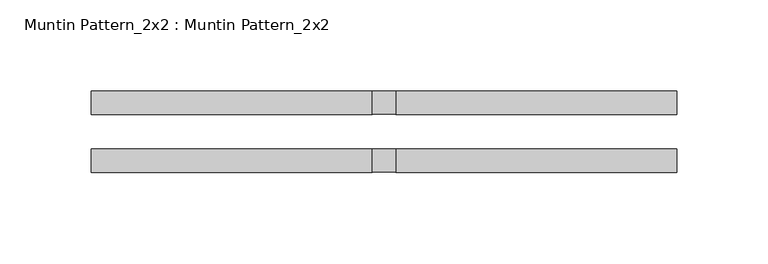
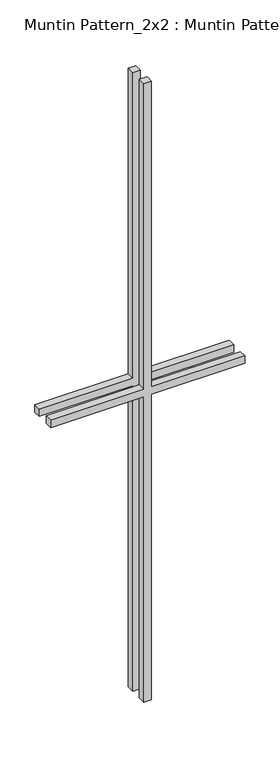
"""IFC4 building model written with IfcOpenShell, lengths in millimetres: proxy geometry, Muntin Pattern_2x2 : Muntin Pattern_2x2."""

from ifc_helpers import new_model, si_unit, frame, origin, place, context, project, spatial, polyline, outline, extrude, source, transform, mapped, element, save


def muntin_pattern_2x2_muntin_pattern_2x2_43d02eee(model_context):
    return source(origin(), model_context, "Body", "SweptSolid", [
        extrude(outline(polyline([(546.1, -6.35), (546.1, -160.3375), (533.4, -160.3375), (533.4, -6.35), (0.0, -6.35), (0.0, 6.35), (533.4, 6.35), (533.4, 160.3375), (546.1, 160.3375), (546.1, 6.35), (1079.5, 6.35), (1079.5, -6.35), (546.1, -6.35)])), frame((0.0, -22.225, 0.0), z_axis=(0.0, 1.0, 0.0), x_axis=(0.0, 0.0, 1.0)), (0.0, 0.0, 1.0), 12.7),
        extrude(outline(polyline([(546.1, -6.35), (546.1, -160.3375), (533.4, -160.3375), (533.4, -6.35), (0.0, -6.35), (0.0, 6.35), (533.4, 6.35), (533.4, 160.3375), (546.1, 160.3375), (546.1, 6.35), (1079.5, 6.35), (1079.5, -6.35), (546.1, -6.35)])), frame((0.0, 9.525, 0.0), z_axis=(0.0, 1.0, 0.0), x_axis=(0.0, 0.0, 1.0)), (0.0, 0.0, 1.0), 12.7),
    ])


if __name__ == "__main__":
    model = new_model("IFC4")
    model_context = context("Model", 3, world=origin())
    ifc_project = project(units=[si_unit("LENGTHUNIT", "METRE", prefix="MILLI")], contexts=[model_context])
    site = spatial("IfcSite", under=ifc_project)
    building = spatial("IfcBuilding", under=site)
    placement = place(None, origin())
    muntin_pattern_2x2_muntin_pattern_2x2_shape = muntin_pattern_2x2_muntin_pattern_2x2_43d02eee(model_context)
    element("IfcBuildingElementProxy", 1, Name="Muntin Pattern_2x2 : Muntin Pattern_2x2", ObjectType="Muntin Pattern_2x2 : Muntin Pattern_2x2", at=placement, inside=building, context=model_context, shape_type="MappedRepresentation", body=[
        mapped(muntin_pattern_2x2_muntin_pattern_2x2_shape, transform((0.0, 0.0, 0.0), x_axis=(1.0, 0.0, 0.0), y_axis=(0.0, 1.0, 0.0), z_axis=(0.0, 0.0, 1.0))),
    ])
    save(model, "model.ifc")

# Revit data of these elements
# Type "Muntin Pattern_2x2 : Muntin Pattern_2x2"
#   Width [instance default] = 4' - 0"
#   Thickness = 0' - 0 1/2"
#   Height [instance default] = 4' - 0"
#   Distance = 0' - 0 3/4"
#   Interior Material [instance default] = none
#   Exterior Material [instance default] = none
#   Default Elevation = 0
# Element 1 (IfcBuildingElementProxy, "Muntin Pattern_2x2 : Muntin Pattern_2x2")
#   Width = 1' - 0 5/8"
#   Height = 3' - 6 1/2"
#   Interior Material = Wood - Stained
#   Materials on its faces: "Wood - Stained"
# Materials
#   "Wood - Stained": class "Wood", colour RGB 224 178 126, transparency 0, Cost = 0
